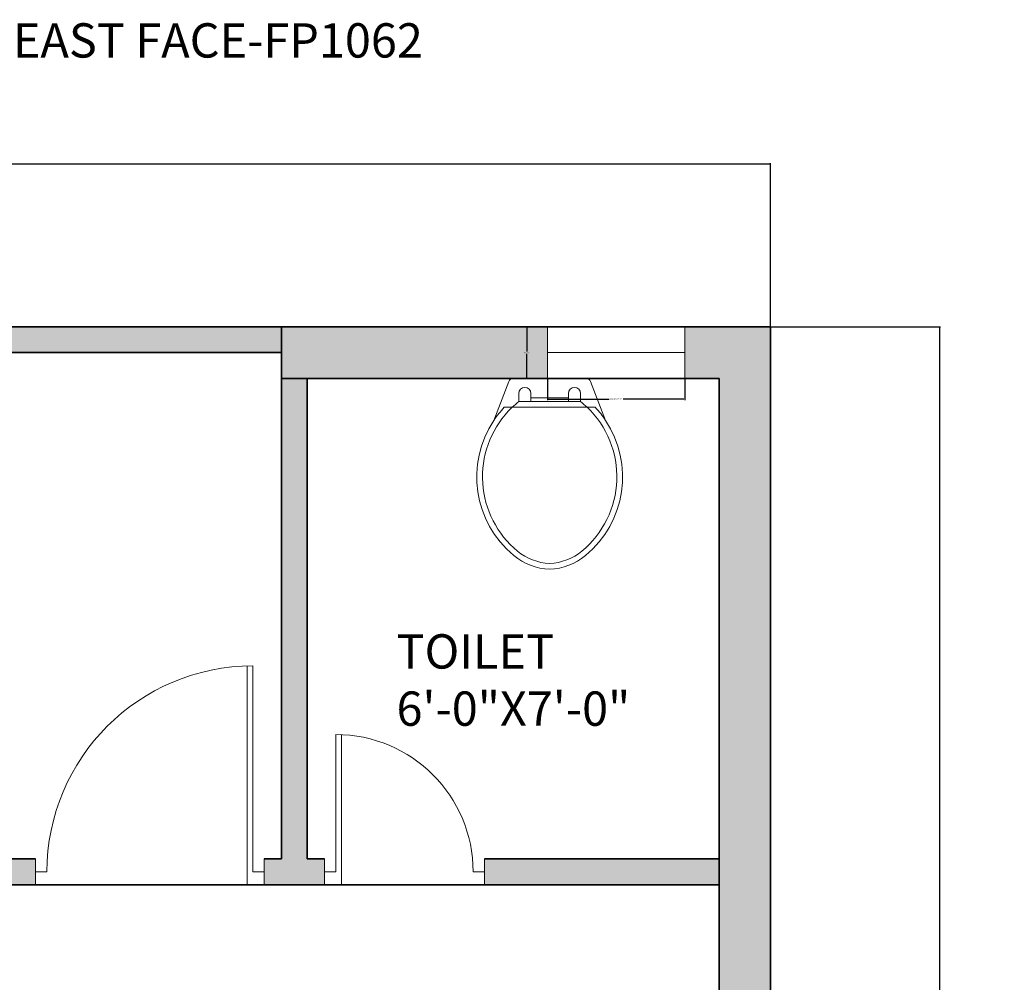
# Model space of a CAD drawing. Units: inches. Extents: x -15 to 423, y -713 to 71.
# Tile 24 of 24: x 251 to 423, y -97 to 71. Entities that reach past the tile are written whole.
import ezdxf

# ---------------------------------------------------------------- set-up
doc = ezdxf.new("R2010")
doc.units = ezdxf.units.IN
doc.header["$MEASUREMENT"] = 0
for name, color, linetype, lineweight in [('A-ANNO-DIMS', 2, 'Continuous', 18), ('A-ANNO-TEXT', 7, 'Continuous', 18), ('A-AREA-IDEN', 7, 'Continuous', 18), ('A-DOOR', 3, 'Continuous', 18), ('A-GLAZ', 5, 'Continuous', 18), ('A-WALL', 7, 'Continuous', 35), ('A-WALL-PATT', 8, 'Continuous', 13), ('WC-Detail_dwgmodels.com', 251, 'Continuous', 13), ('WC-Outline_dwgmodels.com', 250, 'Continuous', 18)]:
    doc.layers.add(name, color=color, linetype=linetype, lineweight=lineweight)
doc.styles.get("Standard").update_dxf_attribs({"font": 'arial.ttf'})
doc.dimstyles.get("Standard").update_dxf_attribs({"dimtxt": 0.18, "dimasz": 0.18, "dimexe": 0.18, "dimexo": 0.0625, "dimgap": 0.09, "dimtad": 0, "dimtih": 1, "dimtoh": 1, "dimdec": 0, "dimzin": 0, "dimdsep": 46, "dimlunit": 3, "dimtxsty": 'Standard', "dimcen": 0.09, "dimadec": 0, "dimazin": 0, "dimtfac": 1, "dimtdec": 0, "dimtofl": 0, "dimtmove": 0, "dimatfit": 3, "dimfxl": 1, "dimtolj": 1, "dimtzin": 0, "dimarcsym": 0})

# ---------------------------------------------------------------- blocks, each defined once
blk = doc.blocks.new('*D7')
at = {"layer": 'A-ANNO-DIMS', "color": 0, "lineweight": -2, "transparency": 16777216}
for p, q in [((25.08, 17.56), (25.08, 46.15)), ((25.26, 45.97), (193.13, 45.97)), ((381.9, 45.97), (214.03, 45.97)), ((382.08, 17.56), (382.08, 46.15))]:
    blk.add_line(p, q, dxfattribs=at)
at = {"layer": 'A-ANNO-DIMS', "color": 0, "transparency": 16777216}
for points in [[(25.26, 46), (25.26, 45.94), (25.08, 45.97)], [(381.9, 46), (381.9, 45.94), (382.08, 45.97)]]:
    blk.add_solid(points, dxfattribs=at)
at = {"layer": 'Defpoints', "color": 0, "transparency": 16777216}
for p in [(25.08, 45.97), (25.08, 17.5), (382.08, 17.5)]:
    blk.add_point(p, dxfattribs=at)
at = {"layer": 'A-ANNO-DIMS', "color": 0, "transparency": 16777216, "insert": (203.58, 45.97), "char_height": 6, "attachment_point": 5}
blk.add_mtext('\\A1;29\'-9"', dxfattribs=at)
blk = doc.blocks.new('*D9')
at = {"layer": 'A-ANNO-DIMS', "color": 0, "lineweight": -2, "transparency": 16777216}
for p, q in [((382.14, 17.5), (411.79, 17.5)), ((411.61, 17.32), (411.61, -324.61)), ((411.61, -672.82), (411.61, -330.89)), ((382.14, -673), (411.79, -673))]:
    blk.add_line(p, q, dxfattribs=at)
at = {"layer": 'A-ANNO-DIMS', "color": 0, "transparency": 16777216}
for points in [[(411.58, 17.32), (411.64, 17.32), (411.61, 17.5)], [(411.58, -672.82), (411.64, -672.82), (411.61, -673)]]:
    blk.add_solid(points, dxfattribs=at)
at = {"layer": 'Defpoints', "color": 0, "transparency": 16777216}
for p in [(382.08, 17.5), (382.08, -673), (411.61, -673)]:
    blk.add_point(p, dxfattribs=at)
at = {"layer": 'A-ANNO-DIMS', "color": 0, "transparency": 16777216, "insert": (411.61, -327.75), "char_height": 6, "attachment_point": 5}
blk.add_mtext('\\A1;57\'-7"', dxfattribs=at)
blk = doc.blocks.new('WINDOW-24IN')
for p, q in [((9, 24), (0, 24)), ((0, 24), (0, 0)), ((4.5, 0), (4.5, 24)), ((9, 0), (9, 24)), ((0, 0), (9, 0))]:
    blk.add_line(p, q)
blk = doc.blocks.new('DOOR-24IN-JAMB4_5')
for p, q in [((25, 0), (25, 26.25)), ((26, 2.25), (26, 26.25)), ((0, 2.25), (0, 4.5)), ((28, 4.5), (28, 0)), ((2, 2.25), (0, 2.25)), ((0, 2.25), (0, 0)), ((28, 2.25), (26, 2.25))]:
    blk.add_line(p, q)
blk.add_arc((26, 2.25), 24, 90, 180)
blk = doc.blocks.new('DOOR-36IN-JAMB4_5')
for p, q in [((2, 2.25), (2, 38.25)), ((3, 0), (3, 38.25)), ((0, 4.5), (0, 0)), ((40, 2.25), (40, 4.5)), ((0, 2.25), (2, 2.25)), ((38, 2.25), (40, 2.25)), ((40, 2.25), (40, 0))]:
    blk.add_line(p, q)
blk.add_arc((2, 2.25), 36, 0, 90)
blk = doc.blocks.new('*D23')
at = {"layer": 'A-ANNO-DIMS', "color": 0, "lineweight": -2, "transparency": 16777216}
for p, q in [((343.09, 8.44), (343.09, 4.72)), ((367.09, 8.44), (367.09, 4.72)), ((343.27, 4.9), (353.86, 4.9)), ((366.91, 4.9), (356.32, 4.9))]:
    blk.add_line(p, q, dxfattribs=at)
at = {"layer": 'A-ANNO-DIMS', "color": 0, "transparency": 16777216}
for points in [[(343.27, 4.93), (343.27, 4.87), (343.09, 4.9)], [(366.91, 4.93), (366.91, 4.87), (367.09, 4.9)]]:
    blk.add_solid(points, dxfattribs=at)
at = {"layer": 'Defpoints', "color": 0, "transparency": 16777216}
for p in [(343.09, 8.5), (367.09, 8.5), (367.09, 4.9)]:
    blk.add_point(p, dxfattribs=at)
at = {"layer": 'A-ANNO-DIMS', "color": 0, "transparency": 16777216, "insert": (355.09, 4.9), "char_height": 0.18, "attachment_point": 5}
blk.add_mtext('\\A1;WINDOW 2\'-0" TYP.', dxfattribs=at)
blk = doc.blocks.new('*D24')
at = {"layer": 'A-ANNO-DIMS', "color": 0, "lineweight": -2, "transparency": 16777216}
for p, q in [((343.03, 17.5), (339.31, 17.5)), ((339.49, 17.32), (339.49, 13.18)), ((339.49, 8.68), (339.49, 12.82)), ((343.03, 8.5), (339.31, 8.5))]:
    blk.add_line(p, q, dxfattribs=at)
at = {"layer": 'A-ANNO-DIMS', "color": 0, "transparency": 16777216}
for points in [[(339.46, 17.32), (339.52, 17.32), (339.49, 17.5)], [(339.46, 8.68), (339.52, 8.68), (339.49, 8.5)]]:
    blk.add_solid(points, dxfattribs=at)
at = {"layer": 'Defpoints', "color": 0, "transparency": 16777216}
for p in [(343.09, 17.5), (339.49, 8.5), (343.09, 8.5)]:
    blk.add_point(p, dxfattribs=at)
at = {"layer": 'A-ANNO-DIMS', "color": 0, "transparency": 16777216, "insert": (339.49, 13), "char_height": 0.18, "attachment_point": 5}
blk.add_mtext('\\A1;0\'-9" TYP.', dxfattribs=at)

msp = doc.modelspace()

# ---------------------------------------------------------------- hatches: boundary and pattern name
at = {"layer": 'A-WALL-PATT'}
h = msp.add_hatch(color=256, dxfattribs=at)
h.dxf.hatch_style = 1
h.paths.add_polyline_path([(34.08, -349.58), (25.08, -349.58), (25.08, -431), (34.08, -431)])
h.paths.add_polyline_path([(34.08, -467), (25.08, -467), (25.08, -673), (34.08, -673)])
h.paths.add_polyline_path([(373.08, -668.5), (182.08, -668.5), (182.08, -673), (373.08, -673)])
h.paths.add_polyline_path([(253.2, -597.5), (191.08, -597.5), (191.08, -594.5), (182.08, -594.5), (182.08, -606.5), (253.2, -606.5)])
h.paths.add_polyline_path([(373.08, -597.5), (313.2, -597.5), (313.2, -606.5), (373.08, -606.5)])
h.paths.add_polyline_path([(382.08, -545.55), (373.08, -545.55), (373.08, -673), (382.08, -673)])
h.paths.add_polyline_path([(139.08, -488), (34.08, -488), (34.08, -497), (139.08, -497), (139.08, -492.5)])
h.paths.add_polyline_path([(139.08, -396.5), (128.58, -396.5), (128.58, -352.79), (124.08, -352.79), (124.08, -396.5), (34.08, -396.5), (34.08, -410), (139.08, -410), (139.08, -403.25)])
h.paths.add_polyline_path([(191.08, -396.5), (179.08, -396.5), (179.08, -410), (182.08, -410), (182.08, -488), (179.08, -488), (179.08, -497), (182.08, -497), (182.08, -501.43), (191.08, -501.43)])
h.paths.add_polyline_path([(373.08, -396.5), (253.08, -396.5), (253.08, -393.5), (248.58, -393.5), (248.58, -401), (284.58, -401), (284.58, -404), (289.08, -404), (289.08, -401), (373.08, -401)])
h.paths.add_polyline_path([(373.08, -449), (289.08, -449), (289.08, -432), (286.83, -432), (284.58, -432), (284.58, -453.5), (373.08, -453.5)])
h.paths.add_polyline_path([(382.08, -344.27), (373.08, -344.27), (373.08, -413.68), (382.08, -413.68)])
h.paths.add_polyline_path([(382.08, -437.68), (373.08, -437.68), (373.08, -485.55), (382.08, -485.55)])
h.paths.add_polyline_path([(34.08, -188.26), (25.08, -188.26), (25.08, -289.58), (34.08, -289.58)])
h.paths.add_polyline_path([(164.08, -236), (34.08, -236), (34.08, -240.5), (124.08, -240.5), (124.08, -293.12), (128.58, -293.12), (128.58, -240.5), (164.08, -240.5), (164.08, -238.25)])
h.paths.add_polyline_path([(373.08, -236), (242.58, -236), (242.58, -238.25), (242.58, -240.5), (248.58, -240.5), (248.58, -353.5), (250.83, -353.5), (253.08, -353.5), (253.08, -240.5), (373.08, -240.5)])
h.paths.add_polyline_path([(382.08, -190.86), (373.08, -190.86), (373.08, -284.27), (382.08, -284.27)])
h.paths.add_polyline_path([(211.58, -80), (253.58, -80), (253.58, -77.75), (253.58, -75.5), (153.58, -75.5), (153.58, -77.75), (153.58, -80), (207.08, -80), (207.08, -236), (204.08, -236), (204.08, -240.5), (214.58, -240.5), (214.58, -236), (211.58, -236)])
h.paths.add_polyline_path([(34.08, 8.5), (70.36, 8.5), (70.36, 17.5), (25.08, 17.5), (25.08, -128.26), (34.08, -128.26)])
h.paths.add_polyline_path([(110.58, 17.5), (94.36, 17.5), (94.36, 8.5), (110.58, 8.5)])
h.paths.add_polyline_path([(296.58, 17.5), (110.58, 17.5), (110.58, 13), (296.58, 13)])
h.paths.add_polyline_path([(110.58, 8.5), (106.08, 8.5), (106.08, -75.5), (103.08, -75.5), (103.08, -80), (113.58, -80), (113.58, -77.75), (113.58, -75.5), (110.58, -75.5)])
h.paths.add_polyline_path([(75.08, -75.5), (34.08, -75.5), (34.08, -80), (75.08, -80), (75.08, -77.75)])
h.paths.add_polyline_path([(343.09, 17.5), (296.58, 17.5), (296.58, 13), (296.58, 8.5), (343.09, 8.5)])
h.paths.add_polyline_path([(304.08, -75.5), (301.08, -75.5), (301.08, 8.5), (296.58, 8.5), (296.58, -75.5), (293.58, -75.5), (293.58, -80), (304.08, -80)])
h.paths.add_polyline_path([(382.08, 17.5), (367.09, 17.5), (367.09, 8.5), (373.08, 8.5), (373.08, -130.86), (382.08, -130.86)])
h.paths.add_polyline_path([(373.08, -75.5), (332.08, -75.5), (332.08, -77.75), (332.08, -80), (373.08, -80)])

# ---------------------------------------------------------------- linework, layer by layer
at = {"layer": 'A-WALL'}
for p, q in [((25.08, 17.5), (382.08, 17.5)), ((296.58, 17.5), (296.58, -75.5)), ((382.08, 17.5), (382.08, -673)), ((110.58, 13), (296.58, 13)), ((296.58, 8.5), (373.08, 8.5)), ((301.08, 8.5), (301.08, -75.5)), ((373.08, 8.5), (373.08, -673)), ((153.58, -75.5), (253.58, -75.5)), ((293.58, -75.5), (296.58, -75.5)), ((301.08, -75.5), (304.08, -75.5)), ((332.08, -75.5), (373.08, -75.5)), ((211.58, -80), (373.08, -80))]:
    msp.add_line(p, q, dxfattribs=at)
at = {"layer": 'WC-Detail_dwgmodels.com'}
for p, q in [((335.5, 3.45), (336.9, 3.45)), ((350.02, 3.45), (351.42, 3.45))]:
    msp.add_line(p, q, dxfattribs=at)
for points in [[(338.05, 4.46), (338.05, 5.86, -1), (340.18, 5.86), (340.18, 5.13)], [(348.87, 4.46), (348.87, 5.86, 1), (346.74, 5.86), (346.74, 5.13)], [(335.5, 3.45, 0.040937), (333.69, 1.16, 0.163732)], [(338.05, 4.46, 0.022712), (336.9, 3.45, 0.162618)], [(343.46, 4.46), (338.05, 4.46, 0.022712)], [(343.46, 4.46), (348.87, 4.46, -0.476108)], [(348.87, 4.46, -0.022712), (350.02, 3.45, -0.162618)], [(351.42, 3.45, -0.040937), (353.23, 1.16, -0.163732)]]:
    msp.add_lwpolyline(points, format="xyb", dxfattribs=at)
for points in [[(346.74, 5.13), (340.18, 5.13)], [(340.18, 5.13), (340.18, 4.46)], [(346.74, 5.13), (346.74, 4.46)]]:
    msp.add_lwpolyline(points, dxfattribs=at)
at = {"layer": 'WC-Outline_dwgmodels.com'}
for p in [(336.9, 3.45), (350.02, 3.45)]:
    msp.add_line(p, (343.46, 3.45), dxfattribs=at)
for points in [[(343.46, 8.5), (337.09, 8.5, 0.31031), (336.31, 7.96), (333.69, 1.16, 0.209071)], [(343.46, 8.5), (349.83, 8.5, -0.31031), (350.61, 7.96), (353.23, 1.16, -0.209071)], [(336.9, 3.45, 0.014165), (336.23, 2.77, 0.162618)], [(350.02, 3.45, -0.448546), (349.09, -21.68, -0.162618), (343.46, -23.85, -0.470877)], [(336.23, 2.77, 0.431639), (337.83, -21.68, 0.162618), (343.46, -23.85, 0.470877)], [(333.69, 1.16, 0.383919), (337.19, -22.45, 0.163732), (343.46, -24.85, 0.359733)], [(353.23, 1.16, -0.383919), (349.73, -22.45, -0.163732), (343.46, -24.85, -0.359733)]]:
    msp.add_lwpolyline(points, format="xyb", dxfattribs=at)

# ---------------------------------------------------------------- block references
at = {"layer": 'A-DOOR', "extrusion": (0, 0, -1), "zscale": -1}
for name, p in [('DOOR-36IN-JAMB4_5', (-293.58, -80)), ('DOOR-24IN-JAMB4_5', (-332.08, -80))]:
    msp.add_blockref(name, p, dxfattribs=at)
at = {"layer": 'A-GLAZ', "rotation": 269.9999999999998}
msp.add_blockref('WINDOW-24IN', (343.09, 17.5), dxfattribs=at)

# ---------------------------------------------------------------- texts
at = {"layer": 'A-ANNO-TEXT', "insert": (133.75, 70.58), "char_height": 6, "attachment_point": 1}
msp.add_mtext('30X60[1800sq ft]HOUSE PLAN-EAST FACE-FP1062', dxfattribs=at)
at = {"layer": 'A-AREA-IDEN', "insert": (316.69, -36.22), "char_height": 6, "attachment_point": 1}
msp.add_mtext('TOILET\\P6\'-0"X7\'-0"', dxfattribs=at)

# ---------------------------------------------------------------- dimensions: what is measured, and where the dimension line sits
at = {"layer": 'A-ANNO-DIMS'}
dim = msp.add_linear_dim(base=(25.08, 45.97), p1=(382.08, 17.5), p2=(25.08, 17.5), dimstyle='Standard', override={"dimtxt": 6, "dimclrd": 0, "dimclre": 0, "dimclrt": 0}, dxfattribs=at)
dim.commit()
dim.dimension.update_dxf_attribs({"geometry": '*D7', "text_midpoint": (203.58, 45.97)})
dim = msp.add_linear_dim(base=(339.49, 8.5), p1=(343.09, 17.5), p2=(343.09, 8.5), angle=270, text='<> TYP.', dimstyle='Standard', override={"dimdec": 1, "dimlfac": 1, "dimrnd": 0, "dimzin": 1, "dimdsep": 46, "dimlunit": 4, "dimfrac": 2}, dxfattribs=at)
dim.commit()
dim.dimension.update_dxf_attribs({"geometry": '*D24', "text_midpoint": (339.49, 13)})
dim = msp.add_linear_dim(base=(411.6050599, -672.99989936), p1=(382.08055573, 17.50010064), p2=(382.08055573, -672.99989936), angle=90, dimstyle='Standard', override={"dimtxt": 6, "dimclrd": 0, "dimclre": 0, "dimclrt": 0}, dxfattribs=at)
dim.commit()
dim.dimension.update_dxf_attribs({"geometry": '*D9', "text_midpoint": (411.6050599, -327.74989936)})
dim = msp.add_linear_dim(base=(367.09, 4.9), p1=(343.09, 8.5), p2=(367.09, 8.5), text='WINDOW <> TYP.', dimstyle='Standard', override={"dimdec": 1, "dimlfac": 1, "dimrnd": 0, "dimzin": 1, "dimdsep": 46, "dimlunit": 4, "dimfrac": 2}, dxfattribs=at)
dim.commit()
dim.dimension.update_dxf_attribs({"geometry": '*D23', "text_midpoint": (355.09, 4.9)})

doc.saveas('drawing.dxf')
